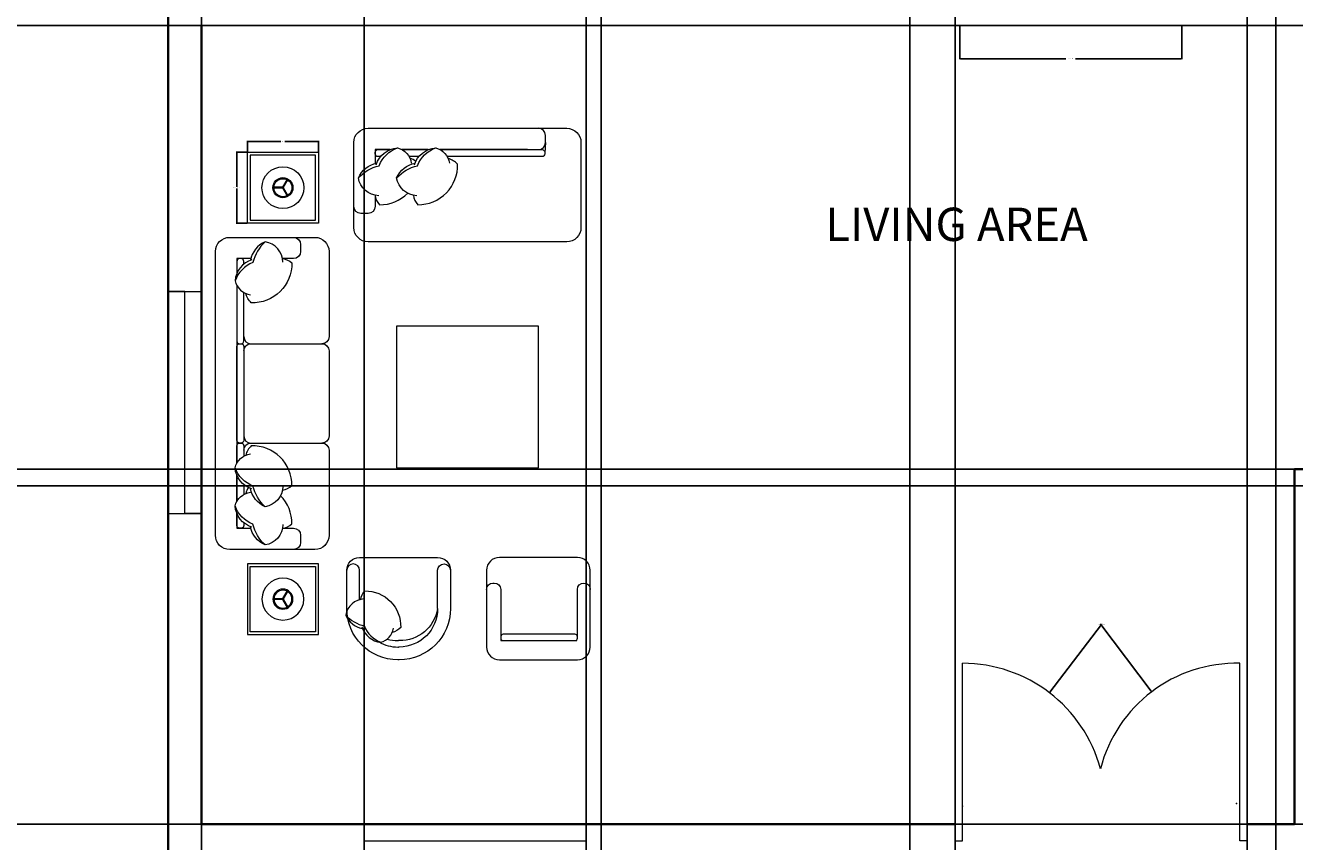
# Model space of a CAD drawing. Units: inches. Extents: x 1770 to 2988, y 1161 to 3221.
# Tile 8 of 44: x 2113 to 2456, y 1614 to 1835. Entities that reach past the tile are written whole.
import ezdxf

# ---------------------------------------------------------------- set-up
doc = ezdxf.new("R2010")
doc.units = ezdxf.units.IN
for name, color, linetype, lineweight in [('A-ANNO-DIMS', 2, 'Continuous', 18), ('A-AREA-IDEN', 7, 'Continuous', 18), ('A-DOOR', 4, 'Continuous', 18), ('A-FURN', 8, 'Continuous', 13), ('A-GLAZ', 4, 'Continuous', 18), ('A-WALL', 7, 'Continuous', 35)]:
    doc.layers.add(name, color=color, linetype=linetype, lineweight=lineweight)
doc.styles.get("Standard").update_dxf_attribs({"font": 'arial.ttf'})
doc.dimstyles.get("Standard").update_dxf_attribs({"dimtxt": 0.18, "dimasz": 0.18, "dimexe": 0.18, "dimexo": 0.0625, "dimgap": 0.09, "dimtad": 0, "dimtih": 1, "dimtoh": 1, "dimdec": 4, "dimzin": 0, "dimdsep": 46, "dimtxsty": 'Standard', "dimcen": 0.09, "dimadec": 0, "dimazin": 0, "dimtfac": 1, "dimtdec": 4, "dimtofl": 0, "dimtmove": 0, "dimatfit": 3, "dimfxl": 1, "dimtolj": 1, "dimtzin": 0, "dimarcsym": 0})

# ---------------------------------------------------------------- blocks, each defined once
blk = doc.blocks.new('TABLE-END-WITH-LAMP')
for p, q in [((9.49, 9.65), (10.84, 12)), ((9.7, 9.53), (11.05, 11.88)), ((9.59, 9.71), (6.89, 9.71)), ((9.59, 9.47), (6.89, 9.47)), ((9.49, 9.53), (10.84, 7.19)), ((9.7, 9.65), (11.05, 7.31))]:
    blk.add_line(p, q)
at = {"ltscale": 0.03}
blk.add_lwpolyline([(19.19, 19.19), (19.19, 0), (0, 0), (0, 19.19)], close=True, dxfattribs=at)
blk.add_lwpolyline([(18.42, 0.77), (18.42, 18.42), (0.77, 18.42), (0.77, 0.77)], close=True)
for radius in [5.66, 2.71, 2.43]:
    blk.add_circle((9.59, 9.59), radius)
blk = doc.blocks.new('WIN-60-EXT')
for p, q in [((0, 9), (0, 0)), ((60, 4.5), (60, 9)), ((60, 9), (60, 0)), ((0, 0), (0, 4.5)), ((0, 4.5), (60, 4.5))]:
    blk.add_line(p, q)
blk = doc.blocks.new('*D34')
at = {"layer": 'A-ANNO-DIMS', "color": 0, "lineweight": -2, "transparency": 16777216}
for p, q in [((2365.67, 1835.14), (2365.67, 1826.02)), ((2425.67, 1835.14), (2425.67, 1826.02)), ((2365.85, 1826.2), (2394.35, 1826.2)), ((2425.49, 1826.2), (2397, 1826.2))]:
    blk.add_line(p, q, dxfattribs=at)
at = {"layer": 'A-ANNO-DIMS', "color": 0, "transparency": 16777216}
for points in [[(2365.85, 1826.23), (2365.85, 1826.17), (2365.67, 1826.2)], [(2425.49, 1826.23), (2425.49, 1826.17), (2425.67, 1826.2)]]:
    blk.add_solid(points, dxfattribs=at)
at = {"layer": 'Defpoints', "color": 0, "transparency": 16777216}
for p in [(2365.67, 1835.2), (2425.67, 1835.2), (2425.67, 1826.2)]:
    blk.add_point(p, dxfattribs=at)
at = {"layer": 'A-ANNO-DIMS', "color": 0, "transparency": 16777216, "insert": (2395.67, 1826.2), "char_height": 0.18, "attachment_point": 5}
blk.add_mtext('\\A1;COURT WIN. 60 TYP.', dxfattribs=at)
blk = doc.blocks.new('*D42')
at = {"layer": 'A-ANNO-DIMS', "color": 0, "lineweight": -2, "transparency": 16777216}
for p, q in [((2173.03, 1800.91), (2170.03, 1800.91)), ((2170.21, 1800.73), (2170.21, 1791.5)), ((2170.21, 1781.9), (2170.21, 1791.13)), ((2173.03, 1781.72), (2170.03, 1781.72))]:
    blk.add_line(p, q, dxfattribs=at)
at = {"layer": 'A-ANNO-DIMS', "color": 0, "transparency": 16777216}
for points in [[(2170.18, 1800.73), (2170.24, 1800.73), (2170.21, 1800.91)], [(2170.18, 1781.9), (2170.24, 1781.9), (2170.21, 1781.72)]]:
    blk.add_solid(points, dxfattribs=at)
at = {"layer": 'Defpoints', "color": 0, "transparency": 16777216}
for p in [(2170.21, 1800.91), (2173.09, 1800.91), (2173.09, 1781.72)]:
    blk.add_point(p, dxfattribs=at)
at = {"layer": 'A-ANNO-DIMS', "color": 0, "transparency": 16777216, "insert": (2170.21, 1791.31), "char_height": 0.18, "attachment_point": 5}
blk.add_mtext('\\A1;END TABLE 19 TYP.', dxfattribs=at)
blk = doc.blocks.new('*D43')
at = {"layer": 'A-ANNO-DIMS', "color": 0, "lineweight": -2, "transparency": 16777216}
for p, q in [((2173.09, 1800.97), (2173.09, 1803.96)), ((2173.27, 1803.78), (2182.16, 1803.78)), ((2192.09, 1803.78), (2183.2, 1803.78)), ((2192.27, 1800.97), (2192.27, 1803.96))]:
    blk.add_line(p, q, dxfattribs=at)
at = {"layer": 'A-ANNO-DIMS', "color": 0, "transparency": 16777216}
for points in [[(2173.27, 1803.81), (2173.27, 1803.75), (2173.09, 1803.78)], [(2192.09, 1803.81), (2192.09, 1803.75), (2192.27, 1803.78)]]:
    blk.add_solid(points, dxfattribs=at)
at = {"layer": 'Defpoints', "color": 0, "transparency": 16777216}
for p in [(2192.27, 1803.78), (2173.09, 1800.91), (2192.27, 1800.91)]:
    blk.add_point(p, dxfattribs=at)
at = {"layer": 'A-ANNO-DIMS', "color": 0, "transparency": 16777216, "insert": (2182.68, 1803.78), "char_height": 0.18, "attachment_point": 5}
blk.add_mtext('\\A1;19 TYP.', dxfattribs=at)
blk = doc.blocks.new('*D63')
at = {"layer": 'A-ANNO-DIMS', "color": 0, "lineweight": -2, "transparency": 16777216}
for p, q in [((2352.17, 1323.59), (2352.17, 2570.7)), ((2352.35, 2570.52), (2401.24, 2570.52)), ((2450.91, 2570.52), (2402.02, 2570.52)), ((2451.09, 1323.59), (2451.09, 2570.7))]:
    blk.add_line(p, q, dxfattribs=at)
at = {"layer": 'A-ANNO-DIMS', "color": 0, "transparency": 16777216}
for points in [[(2352.35, 2570.55), (2352.35, 2570.49), (2352.17, 2570.52)], [(2450.91, 2570.55), (2450.91, 2570.49), (2451.09, 2570.52)]]:
    blk.add_solid(points, dxfattribs=at)
at = {"layer": 'Defpoints', "color": 0, "transparency": 16777216}
for p in [(2451.09, 2570.52), (2352.17, 1323.53), (2451.09, 1323.53)]:
    blk.add_point(p, dxfattribs=at)
at = {"layer": 'A-ANNO-DIMS', "color": 0, "transparency": 16777216, "insert": (2401.63, 2570.52), "char_height": 0.18, "attachment_point": 5}
blk.add_mtext('\\A1;98.93', dxfattribs=at)
blk = doc.blocks.new('*D70')
at = {"layer": 'A-ANNO-DIMS', "color": 0, "lineweight": -2, "transparency": 16777216}
for p, q in [((2160.7, 2171.14), (2160.7, 1165.57)), ((2268.7, 2171.14), (2268.7, 1165.57)), ((2160.88, 1165.75), (2214.42, 1165.75)), ((2268.52, 1165.75), (2214.98, 1165.75))]:
    blk.add_line(p, q, dxfattribs=at)
at = {"layer": 'A-ANNO-DIMS', "color": 0, "transparency": 16777216}
for points in [[(2160.88, 1165.78), (2160.88, 1165.72), (2160.7, 1165.75)], [(2268.52, 1165.78), (2268.52, 1165.72), (2268.7, 1165.75)]]:
    blk.add_solid(points, dxfattribs=at)
at = {"layer": 'Defpoints', "color": 0, "transparency": 16777216}
for p in [(2160.7, 2171.2), (2268.7, 2171.2), (2268.7, 1165.75)]:
    blk.add_point(p, dxfattribs=at)
at = {"layer": 'A-ANNO-DIMS', "color": 0, "transparency": 16777216, "insert": (2214.7, 1165.75), "char_height": 0.18, "attachment_point": 5}
blk.add_mtext('\\A1;108', dxfattribs=at)
blk = doc.blocks.new('*D76')
at = {"layer": 'A-ANNO-DIMS', "color": 0, "lineweight": -2, "transparency": 16777216}
for p, q in [((2460.63, 1710.7), (1907.1, 1710.7)), ((1907.28, 1710.52), (1907.28, 1665.13)), ((1907.28, 1619.38), (1907.28, 1664.77)), ((2460.63, 1619.2), (1907.1, 1619.2))]:
    blk.add_line(p, q, dxfattribs=at)
at = {"layer": 'A-ANNO-DIMS', "color": 0, "transparency": 16777216}
for points in [[(1907.25, 1710.52), (1907.31, 1710.52), (1907.28, 1710.7)], [(1907.25, 1619.38), (1907.31, 1619.38), (1907.28, 1619.2)]]:
    blk.add_solid(points, dxfattribs=at)
at = {"layer": 'Defpoints', "color": 0, "transparency": 16777216}
for p in [(1907.28, 1710.7), (2460.7, 1710.7), (2460.7, 1619.2)]:
    blk.add_point(p, dxfattribs=at)
at = {"layer": 'A-ANNO-DIMS', "color": 0, "transparency": 16777216, "insert": (1907.28, 1664.95), "char_height": 0.18, "attachment_point": 5}
blk.add_mtext('\\A1;91.5', dxfattribs=at)
blk = doc.blocks.new('*D78')
at = {"layer": 'A-ANNO-DIMS', "color": 0, "lineweight": -2, "transparency": 16777216}
for p, q in [((2160.63, 1835.2), (1907.1, 1835.2)), ((1907.28, 1835.02), (1907.28, 1727.38)), ((1907.28, 1619.38), (1907.28, 1727.02)), ((2160.63, 1619.2), (1907.1, 1619.2))]:
    blk.add_line(p, q, dxfattribs=at)
at = {"layer": 'A-ANNO-DIMS', "color": 0, "transparency": 16777216}
for points in [[(1907.25, 1835.02), (1907.31, 1835.02), (1907.28, 1835.2)], [(1907.25, 1619.38), (1907.31, 1619.38), (1907.28, 1619.2)]]:
    blk.add_solid(points, dxfattribs=at)
at = {"layer": 'Defpoints', "color": 0, "transparency": 16777216}
for p in [(1907.28, 1835.2), (2160.7, 1835.2), (2160.7, 1619.2)]:
    blk.add_point(p, dxfattribs=at)
at = {"layer": 'A-ANNO-DIMS', "color": 0, "transparency": 16777216, "insert": (1907.28, 1727.2), "char_height": 0.18, "attachment_point": 5}
blk.add_mtext('\\A1;216', dxfattribs=at)
blk = doc.blocks.new('*D79')
at = {"layer": 'A-ANNO-DIMS', "color": 0, "lineweight": -2, "transparency": 16777216}
for p, q in [((2151.7, 1610.26), (2151.7, 2570.7)), ((2151.88, 2570.52), (2177.78, 2570.52)), ((2204.48, 2570.52), (2178.57, 2570.52)), ((2204.66, 1610.26), (2204.66, 2570.7))]:
    blk.add_line(p, q, dxfattribs=at)
at = {"layer": 'A-ANNO-DIMS', "color": 0, "transparency": 16777216}
for points in [[(2151.88, 2570.55), (2151.88, 2570.49), (2151.7, 2570.52)], [(2204.48, 2570.55), (2204.48, 2570.49), (2204.66, 2570.52)]]:
    blk.add_solid(points, dxfattribs=at)
at = {"layer": 'Defpoints', "color": 0, "transparency": 16777216}
for p in [(2204.66, 2570.52), (2151.7, 1610.2), (2204.66, 1610.2)]:
    blk.add_point(p, dxfattribs=at)
at = {"layer": 'A-ANNO-DIMS', "color": 0, "transparency": 16777216, "insert": (2178.18, 2570.52), "char_height": 0.18, "attachment_point": 5}
blk.add_mtext('\\A1;52.96', dxfattribs=at)
blk = doc.blocks.new('*D80')
at = {"layer": 'A-ANNO-DIMS', "color": 0, "lineweight": -2, "transparency": 16777216}
for p, q in [((2264.66, 1610.26), (2264.66, 2570.7)), ((2264.84, 2570.52), (2314.14, 2570.52)), ((2364.23, 2570.52), (2314.93, 2570.52)), ((2364.41, 1610.26), (2364.41, 2570.7))]:
    blk.add_line(p, q, dxfattribs=at)
at = {"layer": 'A-ANNO-DIMS', "color": 0, "transparency": 16777216}
for points in [[(2264.84, 2570.55), (2264.84, 2570.49), (2264.66, 2570.52)], [(2364.23, 2570.55), (2364.23, 2570.49), (2364.41, 2570.52)]]:
    blk.add_solid(points, dxfattribs=at)
at = {"layer": 'Defpoints', "color": 0, "transparency": 16777216}
for p in [(2364.41, 2570.52), (2264.66, 1610.2), (2364.41, 1610.2)]:
    blk.add_point(p, dxfattribs=at)
at = {"layer": 'A-ANNO-DIMS', "color": 0, "transparency": 16777216, "insert": (2314.53, 2570.52), "char_height": 0.18, "attachment_point": 5}
blk.add_mtext('\\A1;99.76', dxfattribs=at)
blk = doc.blocks.new('*D81')
at = {"layer": 'A-ANNO-DIMS', "color": 0, "lineweight": -2, "transparency": 16777216}
for p, q in [((2364.41, 1610.26), (2364.41, 2570.7)), ((2364.59, 2570.52), (2403.51, 2570.52)), ((2443.21, 2570.52), (2404.29, 2570.52)), ((2443.39, 1610.26), (2443.39, 2570.7))]:
    blk.add_line(p, q, dxfattribs=at)
at = {"layer": 'A-ANNO-DIMS', "color": 0, "transparency": 16777216}
for points in [[(2364.59, 2570.55), (2364.59, 2570.49), (2364.41, 2570.52)], [(2443.21, 2570.55), (2443.21, 2570.49), (2443.39, 2570.52)]]:
    blk.add_solid(points, dxfattribs=at)
at = {"layer": 'Defpoints', "color": 0, "transparency": 16777216}
for p in [(2443.39, 2570.52), (2364.41, 1610.2), (2443.39, 1610.2)]:
    blk.add_point(p, dxfattribs=at)
at = {"layer": 'A-ANNO-DIMS', "color": 0, "transparency": 16777216, "insert": (2403.9, 2570.52), "char_height": 0.18, "attachment_point": 5}
blk.add_mtext('\\A1;78.97', dxfattribs=at)
blk = doc.blocks.new('*D82')
at = {"layer": 'A-ANNO-DIMS', "color": 0, "lineweight": -2, "transparency": 16777216}
for p, q in [((2443.39, 1610.26), (2443.39, 2570.7)), ((2443.57, 2570.52), (2486.45, 2570.52)), ((2530.12, 2570.52), (2487.24, 2570.52)), ((2530.3, 1610.26), (2530.3, 2570.7))]:
    blk.add_line(p, q, dxfattribs=at)
at = {"layer": 'A-ANNO-DIMS', "color": 0, "transparency": 16777216}
for points in [[(2443.57, 2570.55), (2443.57, 2570.49), (2443.39, 2570.52)], [(2530.12, 2570.55), (2530.12, 2570.49), (2530.3, 2570.52)]]:
    blk.add_solid(points, dxfattribs=at)
at = {"layer": 'Defpoints', "color": 0, "transparency": 16777216}
for p in [(2530.3, 2570.52), (2443.39, 1610.2), (2530.3, 1610.2)]:
    blk.add_point(p, dxfattribs=at)
at = {"layer": 'A-ANNO-DIMS', "color": 0, "transparency": 16777216, "insert": (2486.85, 2570.52), "char_height": 0.18, "attachment_point": 5}
blk.add_mtext('\\A1;86.92', dxfattribs=at)
blk = doc.blocks.new('*D83')
at = {"layer": 'A-ANNO-DIMS', "color": 0, "lineweight": -2, "transparency": 16777216}
for p, q in [((2513.13, 1835.2), (1907.1, 1835.2)), ((1907.28, 1835.02), (1907.28, 1775.38)), ((1907.28, 1715.38), (1907.28, 1775.02)), ((2513.13, 1715.2), (1907.1, 1715.2))]:
    blk.add_line(p, q, dxfattribs=at)
at = {"layer": 'A-ANNO-DIMS', "color": 0, "transparency": 16777216}
for points in [[(1907.25, 1835.02), (1907.31, 1835.02), (1907.28, 1835.2)], [(1907.25, 1715.38), (1907.31, 1715.38), (1907.28, 1715.2)]]:
    blk.add_solid(points, dxfattribs=at)
at = {"layer": 'Defpoints', "color": 0, "transparency": 16777216}
for p in [(1907.28, 1835.2), (2513.2, 1835.2), (2513.2, 1715.2)]:
    blk.add_point(p, dxfattribs=at)
at = {"layer": 'A-ANNO-DIMS', "color": 0, "transparency": 16777216, "insert": (1907.28, 1775.2), "char_height": 0.18, "attachment_point": 5}
blk.add_mtext('\\A1;120', dxfattribs=at)
blk = doc.blocks.new('*D117')
at = {"layer": 'A-ANNO-DIMS', "color": 0, "lineweight": -2, "transparency": 16777216}
for p, q in [((2404, 1673.15), (2390.01, 1654.88)), ((2404.18, 1673.15), (2404, 1673.15)), ((2366.32, 1624.06), (2366.5, 1624.06)), ((2366.41, 1623.97), (2366.41, 1624.15))]:
    blk.add_line(p, q, dxfattribs=at)
at = {"layer": 'A-ANNO-DIMS', "color": 0, "transparency": 16777216}
blk.add_solid([(2389.99, 1654.9), (2390.04, 1654.87), (2389.9, 1654.74)], dxfattribs=at)
at = {"layer": 'Defpoints', "color": 0, "transparency": 16777216}
for p in [(2389.9, 1654.74), (2366.41, 1624.06)]:
    blk.add_point(p, dxfattribs=at)
at = {"layer": 'A-ANNO-DIMS', "color": 0, "transparency": 16777216, "insert": (2404.66, 1673.15), "char_height": 0.18, "attachment_point": 5}
blk.add_mtext('\\A1;R38.64', dxfattribs=at)
blk = doc.blocks.new('*D118')
at = {"layer": 'A-ANNO-DIMS', "color": 0, "lineweight": -2, "transparency": 16777216}
for p, q in [((2403.62, 1673.15), (2403.8, 1673.15)), ((2403.8, 1673.15), (2417.45, 1655.15)), ((2440.39, 1624.77), (2440.57, 1624.77)), ((2440.48, 1624.68), (2440.48, 1624.86))]:
    blk.add_line(p, q, dxfattribs=at)
at = {"layer": 'A-ANNO-DIMS', "color": 0, "transparency": 16777216}
blk.add_solid([(2417.47, 1655.17), (2417.43, 1655.13), (2417.56, 1655.01)], dxfattribs=at)
at = {"layer": 'Defpoints', "color": 0, "transparency": 16777216}
for p in [(2417.56, 1655.01), (2440.48, 1624.77)]:
    blk.add_point(p, dxfattribs=at)
at = {"layer": 'A-ANNO-DIMS', "color": 0, "transparency": 16777216, "insert": (2403.14, 1673.15), "char_height": 0.18, "attachment_point": 5}
blk.add_mtext('\\A1;R37.94', dxfattribs=at)

msp = doc.modelspace()

# ---------------------------------------------------------------- linework, layer by layer
at = {"layer": 'A-DOOR'}
for p, q in [((2366.4122, 1650.7021), (2366.4122, 1662.7021)), ((2441.3863, 1614.7021), (2441.3863, 1662.7021)), ((2366.4122, 1614.7021), (2366.4122, 1650.7021)), ((2364.4122, 1619.2021), (2364.4122, 1610.2021)), ((2443.3863, 1619.2021), (2443.3863, 1610.2021)), ((2364.4122, 1610.2021), (2364.4122, 1614.7021)), ((2364.4122, 1614.7021), (2366.4122, 1614.7021)), ((2443.3863, 1614.7021), (2441.3863, 1614.7021))]:
    msp.add_line(p, q, dxfattribs=at)
for centre, radius, start, end in [((2366.4122, 1624.0638), 38.6383, 15.114663, 90), ((2440.4817, 1624.7703), 37.9426, 88.633889, 165.705073)]:
    msp.add_arc(centre, radius, start, end, dxfattribs=at)
at = {"layer": 'A-FURN'}
msp.add_line((2253.6667, 1803.5385), (2253.4804, 1800.6607), dxfattribs=at)
at = {"layer": 'A-FURN', "ltscale": 0.03}
for points in [[(2263.2594, 1780.5161, -0.41421356), (2259.4223, 1776.679), (2259.4223, 1776.679, 0.31783725), (2259.4223, 1776.679, -0.41421356), (2259.4223, 1776.679), (2259.4223, 1776.679, 1.18618475), (2259.4223, 1776.679, -0.41421356), (2259.4223, 1776.679), (2205.7033, 1776.679, -0.41421356), (2201.8663, 1780.5161), (2201.8663, 1803.5385, -0.41421356), (2205.7033, 1807.3756), (2259.4223, 1807.3756, -0.41421356), (2263.2594, 1803.5385)], [(2191.3143, 1777.8842, -0.41421356), (2195.1514, 1774.0472), (2195.1514, 1751.0247, -0.41421356), (2193.2329, 1749.1062, -0.41421356), (2195.1514, 1747.1877), (2195.1514, 1724.1652, -0.41421356), (2193.2329, 1722.2467, -0.41421356), (2195.1514, 1720.3282), (2195.1514, 1697.3057, -0.41421356), (2191.3143, 1693.4687), (2168.2919, 1693.4687, -0.41421356), (2164.4548, 1697.3057), (2164.4548, 1774.0472, -0.41421356), (2168.2919, 1777.8842)], [(2262.3085, 1663.6402), (2262.3085, 1663.6402, 0.41421356), (2265.7682, 1667.0999), (2265.7682, 1687.8578, 0.41421356), (2262.3085, 1691.3175), (2262.3085, 1691.3175), (2241.2046, 1691.3175, 0.41421356), (2237.745, 1687.8578), (2237.745, 1667.0999, 0.41421356), (2241.2046, 1663.6402)]]:
    msp.add_lwpolyline(points, format="xyb", close=True, dxfattribs=at)
at = {"layer": 'A-FURN'}
for points in [[(2248.7757, 1801.62), (2251.7482, 1801.62, 0.41421356), (2253.6667, 1803.5385), (2253.6667, 1805.4571, 0.41421356), (2251.7482, 1807.3756)], [(2203.0873, 1793.964, -0.14772988), (2208.6946, 1797.2612, -0.21334276), (2213.6423, 1802.0971, -0.17866181)], [(2209.0859, 1799.7014), (2208.3893, 1799.7014, -0.41421356), (2207.6219, 1800.4689), (2207.6219, 1800.8526, -0.41421356), (2208.3893, 1801.62)], [(2211.6579, 1801.62), (2207.6219, 1801.62), (2207.6219, 1797.8496, -0.41421356)], [(2207.92, 1797.524, -0.30666349), (2213.6423, 1802.0971, -0.30632997), (2217.3805, 1797.9206, 0.87284716)], [(2208.3893, 1801.62), (2211.6579, 1801.62, -0.41421356)], [(2213.4224, 1793.964, -0.14772988), (2219.0297, 1797.2612, -0.21334276), (2223.9773, 1802.0971, -0.17866181)], [(2214.8497, 1801.62), (2221.993, 1801.62, -0.41421356)], [(2218.255, 1797.524, -0.30666349), (2223.9773, 1802.0971, -0.30632997), (2227.7156, 1797.9206, 0.87284716)], [(2225.1848, 1801.62), (2252.713, 1801.62, -0.41421356), (2253.4804, 1800.8526), (2253.4804, 1800.4689, -0.41421356), (2252.713, 1799.7014), (2227.1166, 1799.7014, -0.41421356)], [(2219.421, 1799.7014), (2216.7815, 1799.7014, -0.41421356)], [(2218.6302, 1798.4656, 0.07186538), (2217.0217, 1799.2157, -7.11546429)], [(2217.9528, 1789.2451, 0.16554063), (2219.1397, 1786.7101, 0.42598917), (2229.9145, 1797.7008, 0.12152332), (2227.3568, 1799.2157, -7.11546429)], [(2208.5847, 1789.1281, -0.35677236), (2203.0873, 1793.964, -0.24954205), (2208.0684, 1797.9492, 9.61688035)], [(2218.9198, 1789.1281, -0.35677236), (2213.4224, 1793.964, -0.24954205), (2218.4035, 1797.9492, 9.61688035)], [(2207.6219, 1789.2442), (2207.6219, 1786.2717, -0.41421356), (2205.7033, 1784.3532), (2203.7848, 1784.3532, -0.41421356), (2201.8663, 1786.2717)], [(2207.6177, 1789.2451, 0.16554063), (2208.8046, 1786.7101, 0.20023115), (2216.4205, 1789.7974, 0.12152332)], [(2185.5587, 1777.8842, -0.41421356), (2187.4773, 1775.9657), (2187.4773, 1774.0472, -0.41421356), (2185.5587, 1772.1286), (2182.5862, 1772.1286)], [(2177.8664, 1776.6632, 0.14772988), (2174.5692, 1771.0559, 0.21334276), (2169.7333, 1766.1082)], [(2182.7023, 1771.1658, 0.35677236), (2177.8664, 1776.6632, 0.24954205), (2173.8812, 1771.6821)], [(2174.3064, 1771.8305, 0.30666349), (2169.7333, 1766.1082, 0.30632997), (2173.9098, 1762.37)], [(2172.129, 1770.6646), (2172.129, 1771.3612, 0.41421356), (2171.3616, 1772.1286), (2170.9778, 1772.1286, 0.41421356), (2170.2104, 1771.3612)], [(2170.2104, 1771.3612), (2170.2104, 1768.0926, 0.41253535)], [(2182.5853, 1772.1328, -0.16554063), (2185.1203, 1770.9459, -0.42598917), (2174.1296, 1760.1711, -0.12152332), (2172.6147, 1762.7288)], [(2170.2104, 1764.9008), (2170.2104, 1749.8736, 0.41421356), (2170.9778, 1749.1062), (2171.3616, 1749.1062, 0.41421356), (2172.129, 1749.8736), (2172.129, 1762.969, 0.41265155)], [(2172.129, 1751.0247, 0.41421356), (2174.0475, 1749.1062), (2193.2329, 1749.1062, 0.4152491)], [(2172.129, 1747.1877, -0.41421356), (2174.0475, 1749.1062)], [(2172.129, 1724.1652, 0.41421356), (2174.0475, 1722.2467)], [(2174.3064, 1709.8574, -0.30666349), (2169.7333, 1715.5797, -0.30632997), (2173.9098, 1719.3179)], [(2170.2104, 1716.7872), (2170.2104, 1721.4793, -0.41421356), (2170.9778, 1722.2467), (2171.3616, 1722.2467, -0.41421356), (2172.129, 1721.4793), (2172.129, 1718.719, -0.12631336)], [(2172.129, 1720.3282, -0.41421356), (2174.0475, 1722.2467), (2193.2329, 1722.2467, -0.41732018)], [(2182.5853, 1709.5552, 0.16554063), (2185.1203, 1710.742, 0.42598917), (2174.1296, 1721.5169, 0.12152332), (2172.6147, 1718.9592)], [(2177.8664, 1705.0248, -0.14772988), (2174.5692, 1710.6321, -0.21334276), (2169.7333, 1715.5797)], [(2170.2104, 1706.4521), (2170.2104, 1713.5954, -0.41474665)], [(2174.3064, 1699.5223, -0.30666349), (2169.7333, 1705.2446, -0.30632997), (2173.9098, 1708.9829)], [(2172.129, 1711.0234), (2172.129, 1708.3839, -0.41459885)], [(2173.3648, 1710.2325, 0.07186538), (2172.6147, 1708.6241)], [(2182.7023, 1710.5221, -0.35677236), (2177.8664, 1705.0248, -0.24954205), (2173.8812, 1710.0059)], [(2182.5853, 1699.2201, 0.16554063), (2185.1203, 1700.407, 0.20023115), (2182.033, 1708.0228)], [(2177.8664, 1694.6897, -0.14772988), (2174.5692, 1700.297, -0.21334276), (2169.7333, 1705.2446)], [(2170.2104, 1703.2603), (2170.2104, 1699.2243), (2173.9808, 1699.2243, -0.41435211)], [(2170.2104, 1699.9917), (2170.2104, 1703.2603, -0.41446868)], [(2172.129, 1700.6883), (2172.129, 1699.9917, -0.41421356), (2171.3616, 1699.2243), (2170.9778, 1699.2243, -0.41421356), (2170.2104, 1699.9917)], [(2182.7023, 1700.1871, -0.35677236), (2177.8664, 1694.6897, -0.24954205), (2173.8812, 1699.6708)], [(2182.5862, 1699.2243), (2185.5587, 1699.2243, -0.41421356), (2187.4773, 1697.3057), (2187.4773, 1695.3872, -0.41421356), (2185.5587, 1693.4687)], [(2203.4011, 1679.9042), (2203.4011, 1687.8578, 0.41421356), (2201.6713, 1689.5876), (2201.6713, 1689.5876, 0.41421356), (2199.9414, 1687.8578)], [(2224.505, 1677.4787), (2224.505, 1687.8578, -0.41421356), (2226.2348, 1689.5876), (2226.2348, 1689.5876, -0.41421356), (2227.9647, 1687.8578)], [(2203.7433, 1679.9874, -0.16554063), (2204.8134, 1682.273, -0.42598917), (2214.5285, 1672.3634, -0.12152332), (2212.2223, 1670.9975, 7.11546429)], [(2237.745, 1682.6683, -0.41421356), (2239.4748, 1684.3981), (2239.8208, 1684.3981, -0.41421356), (2241.5506, 1682.6683), (2241.5506, 1679.9882)], [(2262.3085, 1669.8676), (2262.3085, 1682.6683, -0.41421356), (2264.0383, 1684.3981), (2264.0383, 1684.3981, -0.41421356), (2265.7682, 1682.6683)], [(2204.6152, 1680.0929, 0.35677236), (2199.6585, 1675.7326, 0.24954205), (2204.1497, 1672.1394, -9.61688035)], [(2199.6585, 1675.7326, 0.14772988), (2204.7143, 1672.7598, 0.21334276), (2209.1753, 1668.3995, 0.17866181)], [(2224.505, 1677.4788, -0.37271891), (2214.126, 1668.8297), (2213.953, 1668.8297)], [(2224.505, 1677.4788, -0.41421356), (2214.126, 1667.0999), (2213.953, 1667.0999)], [(2204.0158, 1672.5228, 0.30666349), (2209.1753, 1668.3995, 0.30632997), (2212.5458, 1672.1652, -0.87284716)], [(2208.6281, 1668.4688, 0.13059149), (2213.7801, 1667.0999), (2213.953, 1667.0999)], [(2210.8308, 1669.2024, 0.07238424), (2213.7801, 1668.8297), (2213.953, 1668.8297)], [(2249.8093, 1670.5595), (2242.2425, 1670.5595, 0.41421356), (2241.5506, 1669.8676), (2241.5506, 1669.5216, 0.41421356), (2242.2425, 1668.8297)], [(2242.2425, 1668.8297), (2248.0675, 1668.8297, 0.41421356)], [(2248.0675, 1668.8297), (2261.6166, 1668.8297, 0.41421356), (2262.3085, 1669.5216), (2262.3085, 1669.8676, 0.41421356), (2261.6166, 1670.5595), (2249.8093, 1670.5595, 0.41421356)]]:
    msp.add_lwpolyline(points, format="xyb", dxfattribs=at)
for points in [[(2221.993, 1801.62), (2214.8497, 1801.62)], [(2248.7757, 1801.62), (2225.1848, 1801.62)], [(2173.9808, 1772.1286), (2170.2104, 1772.1286), (2170.2104, 1768.0926)], [(2170.2104, 1764.9008), (2170.2104, 1716.7872)], [(2170.2104, 1713.5954), (2170.2104, 1706.4521)], [(2241.5506, 1679.9882), (2241.5506, 1668.8297), (2248.0675, 1668.8297)], [(2248.0675, 1668.8297), (2262.1355, 1668.8297)]]:
    msp.add_lwpolyline(points, dxfattribs=at)
at = {"layer": 'A-FURN', "ltscale": 0.03}
msp.add_lwpolyline([(2251.7482, 1715.5318), (2251.7482, 1753.9025), (2213.3775, 1753.9025), (2213.3775, 1715.5318)], close=True, dxfattribs=at)
at = {"layer": 'A-FURN'}
msp.add_lwpolyline([(2170.2104, 1723.0141), (2170.2104, 1748.3388, -0.41421356), (2170.9778, 1749.1062), (2171.3616, 1749.1062, -0.41421356), (2172.129, 1748.3388), (2172.129, 1723.0141, -0.41421356), (2171.3616, 1722.2467), (2170.9778, 1722.2467, -0.41421356)], format="xyb", close=True, dxfattribs=at)
at = {"layer": 'A-FURN', "ltscale": 0.03}
msp.add_lwpolyline([(2213.953, 1691.3175), (2224.505, 1691.3175, -0.41421356), (2227.9647, 1687.8578), (2227.9647, 1677.4788, -0.41421356), (2214.126, 1663.6402), (2213.953, 1663.6402), (2213.7801, 1663.6402, -0.41421356), (2199.9414, 1677.4788), (2199.9414, 1687.8578, -0.41421356), (2203.4011, 1691.3175), (2213.953, 1691.3175)], format="xyb", dxfattribs=at)
at = {"layer": 'A-WALL'}
for p, q in [((2151.696, 2376.7021), (2151.696, 1610.2021)), ((2160.696, 1835.2021), (2160.696, 1619.2021)), ((2456.196, 1715.2021), (2456.196, 1619.2021)), ((2456.196, 1710.7021), (2456.196, 1715.2021)), ((2456.196, 1715.2021), (2460.696, 1715.2021)), ((2160.696, 1619.2021), (2364.4122, 1619.2021)), ((2443.3863, 1619.2021), (2456.196, 1619.2021))]:
    msp.add_line(p, q, dxfattribs=at)

# ---------------------------------------------------------------- block references
at = {"layer": 'A-FURN'}
msp.add_blockref('TABLE-END-WITH-LAMP', (2173.088, 1781.721), dxfattribs=at)
at = {"layer": 'A-FURN', "extrusion": (0, 0, -1), "zscale": -1, "rotation": 180}
msp.add_blockref('TABLE-END-WITH-LAMP', (-2173.088, 1689.6319), dxfattribs=at)
at = {"layer": 'A-GLAZ', "rotation": 90}
msp.add_blockref('WIN-60-EXT', (2160.6961, 1703.238), dxfattribs=at)
at = {"layer": 'A-GLAZ'}
msp.add_blockref('WIN-60-EXT', (2204.657, 1610.202), dxfattribs=at)

# ---------------------------------------------------------------- texts
at = {"layer": 'A-AREA-IDEN', "insert": (2329.3025, 1785.8984), "char_height": 9, "attachment_point": 1}
msp.add_mtext_dynamic_manual_height_columns('LIVING AREA', width=145.901474, gutter_width=12.5, heights=[0], dxfattribs=at)

# ---------------------------------------------------------------- dimensions: what is measured, and where the dimension line sits
at = {"layer": 'A-ANNO-DIMS'}
for base, p1, p2, override, picture, middle in [((2204.6568, 2570.5247), (2151.696, 1610.2021), (2204.6568, 1610.2021), {"dimdec": 2, "dimlfac": 1, "dimrnd": 0, "dimzin": 0, "dimdsep": 46, "dimlunit": 2}, '*D79', (2178.1764, 2570.5247)), ((2364.4122, 2570.5247), (2264.6568, 1610.2021), (2364.4122, 1610.2021), {"dimdec": 2, "dimlfac": 1, "dimrnd": 0, "dimzin": 0, "dimdsep": 46, "dimlunit": 2}, '*D80', (2314.5345, 2570.5247)), ((2451.0947, 2570.5247), (2352.1672, 1323.5288), (2451.0947, 1323.5288), {"dimdec": 2, "dimlfac": 1, "dimrnd": 0, "dimzin": 0, "dimdsep": 46, "dimlunit": 2}, '*D63', (2401.631, 2570.5247)), ((2443.3863, 2570.5247), (2364.4122, 1610.2021), (2443.3863, 1610.2021), {"dimdec": 2, "dimlfac": 1, "dimrnd": 0, "dimzin": 0, "dimdsep": 46, "dimlunit": 2}, '*D81', (2403.8993, 2570.5247)), ((2530.3038, 2570.5247), (2443.3863, 1610.2021), (2530.3038, 1610.2021), {"dimdec": 2, "dimlfac": 1, "dimrnd": 0, "dimzin": 0, "dimdsep": 46, "dimlunit": 2}, '*D82', (2486.8451, 2570.5247)), ((2268.696, 1165.752), (2160.696, 2171.2021), (2268.696, 2171.2021), {"dimdec": 0, "dimlfac": 1, "dimrnd": 0, "dimzin": 0, "dimdsep": 46, "dimlunit": 2}, '*D70', (2214.696, 1165.752))]:
    dim = msp.add_linear_dim(base=base, p1=p1, p2=p2, dimstyle='Standard', override=override, dxfattribs=at)
    dim.commit()
    dim.dimension.update_dxf_attribs({"geometry": picture, "text_midpoint": middle})
for base, p1, p2, override, picture, middle in [((1907.2844, 1835.2021), (2160.696, 1619.2021), (2160.696, 1835.2021), {"dimdec": 0, "dimlfac": 1, "dimrnd": 0, "dimzin": 0, "dimdsep": 46, "dimlunit": 2}, '*D78', (1907.2844, 1727.2021)), ((1907.2844, 1835.2021), (2513.196, 1715.2021), (2513.196, 1835.2021), {"dimdec": 0, "dimlfac": 1, "dimrnd": 0, "dimzin": 0, "dimdsep": 46, "dimlunit": 2}, '*D83', (1907.2844, 1775.2021)), ((1907.2844, 1710.7021), (2460.696, 1619.2021), (2460.696, 1710.7021), {"dimdec": 1, "dimlfac": 1, "dimrnd": 0, "dimzin": 0, "dimdsep": 46, "dimlunit": 2}, '*D76', (1907.2844, 1664.9521))]:
    dim = msp.add_linear_dim(base=base, p1=p1, p2=p2, angle=90, dimstyle='Standard', override=override, dxfattribs=at)
    dim.commit()
    dim.dimension.update_dxf_attribs({"geometry": picture, "text_midpoint": middle})
for base, p1, p2, text, picture, middle in [((2425.672, 1826.2021), (2365.672, 1835.2021), (2425.672, 1835.2021), 'COURT WIN. <> TYP.', '*D34', (2395.672, 1826.2021)), ((2192.2736, 1803.7845), (2173.0882, 1800.9067), (2192.2736, 1800.9067), '<> TYP.', '*D43', (2182.6809, 1803.7845))]:
    dim = msp.add_linear_dim(base=base, p1=p1, p2=p2, text=text, dimstyle='Standard', override={"dimdec": 0, "dimlfac": 1, "dimrnd": 0, "dimzin": 0, "dimdsep": 46, "dimlunit": 2}, dxfattribs=at)
    dim.commit()
    dim.dimension.update_dxf_attribs({"geometry": picture, "text_midpoint": middle})
dim = msp.add_linear_dim(base=(2170.2104, 1800.9067), p1=(2173.0882, 1781.7213), p2=(2173.0882, 1800.9067), angle=90, text='END TABLE <> TYP.', dimstyle='Standard', override={"dimdec": 0, "dimlfac": 1, "dimrnd": 0, "dimzin": 0, "dimdsep": 46, "dimlunit": 2}, dxfattribs=at)
dim.commit()
dim.dimension.update_dxf_attribs({"geometry": '*D42', "text_midpoint": (2170.2104, 1791.314)})
for center, mpoint, picture, middle in [((2366.4122, 1624.0638), (2389.9031, 1654.7411), '*D117', (2404.6571, 1673.1475)), ((2440.4817, 1624.7703), (2417.5579, 1655.0051), '*D118', (2403.1442, 1673.146))]:
    dim = msp.add_radius_dim(center=center, mpoint=mpoint, dimstyle='Standard', override={"dimdec": 2, "dimlfac": 1, "dimrnd": 0, "dimzin": 0, "dimdsep": 46, "dimlunit": 2}, dxfattribs=at)
    dim.commit()
    dim.dimension.update_dxf_attribs({"geometry": picture, "text_midpoint": middle, "dimtype": 164})

doc.saveas('drawing.dxf')
